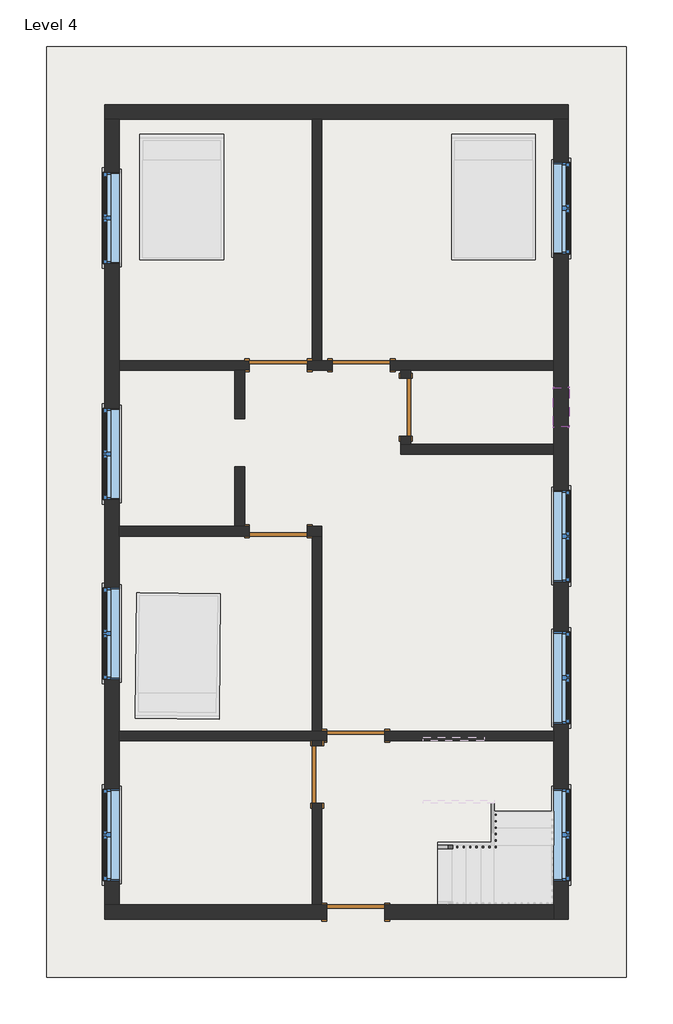
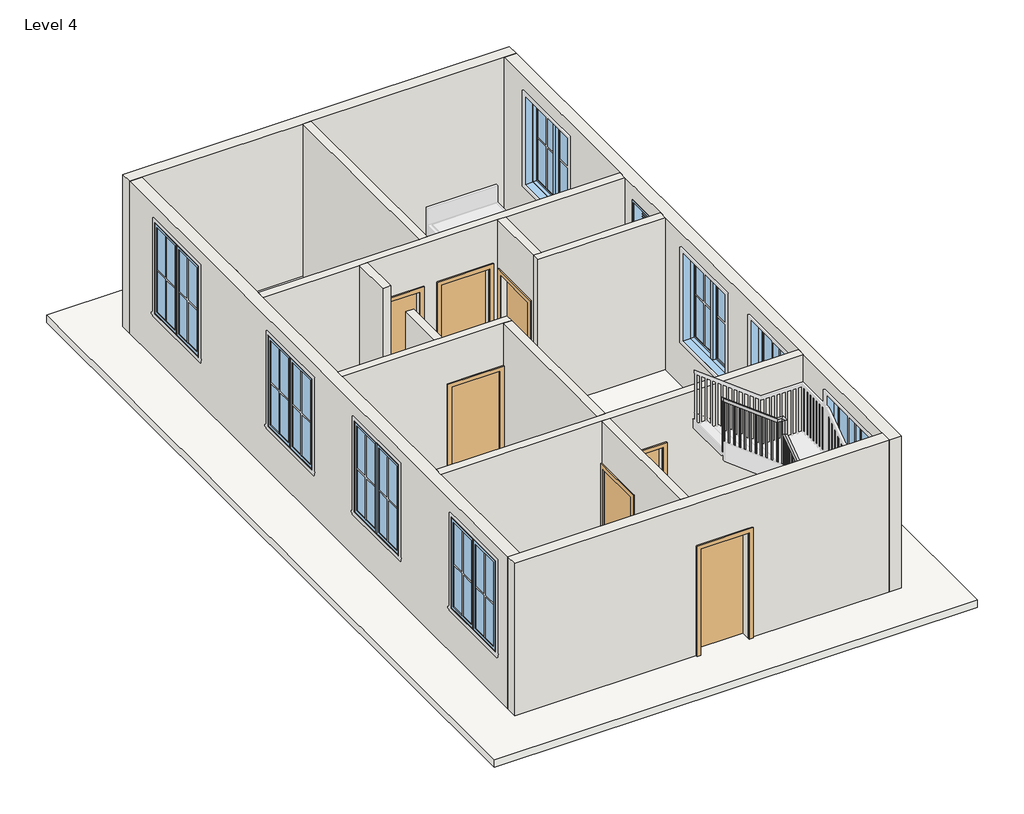
# One storey, part 1 of 2: 14 walls, 9 windows, 7 doors, 1 railing, 1 roof.
"""IFC4 building model written with IfcOpenShell, lengths in millimetres."""

from ifc_helpers import new_model, si_unit, frame, origin, place, context, project, spatial, polyline, outline, extrude, faceted_brep, transform, mapped, element, save
from components import door_2b0b55a0, door_686f89d2, door_16372e1c, door_a90ba1ad, window_9ac97e1a, window_f2d8fef0

model = new_model("IFC4")

# Units and contexts
model_context = context("Model", 3, world=origin())
ifc_project = project(units=[si_unit("LENGTHUNIT", "METRE", prefix="MILLI")], contexts=[model_context])

# Site, building, storey
site = spatial("IfcSite", under=ifc_project)
building = spatial("IfcBuilding", under=site)
storey = spatial("IfcBuildingStorey", under=building, Name="Level 4", Elevation=6400.8)

# Doors
placement = place(None, origin())
door_shape = door_2b0b55a0(model_context)
element("IfcDoor", 1, ObjectType="Single-Flush : 36\" x 80\"", at=placement, inside=storey, context=model_context, shape_type="MappedRepresentation", body=[
    mapped(door_shape, transform((-163.235885, 1707.4649429, 6400.8), x_axis=(0.0, 1.0, 0.0), y_axis=(-1.0, 0.0, 0.0), z_axis=(0.0, 0.0, 1.0))),
])
door_2_shape = door_686f89d2(model_context)
element("IfcDoor", 2, ObjectType="Single-Flush : 36\" x 84\"", at=placement, inside=storey, context=model_context, shape_type="MappedRepresentation", body=[
    mapped(door_2_shape, transform((-861.735885, 2367.8649429, 6400.8), x_axis=(-1.0, 0.0, 0.0), y_axis=(0.0, -1.0, 0.0), z_axis=(0.0, 0.0, 1.0))),
])
element("IfcDoor", 3, ObjectType="Single-Flush : 36\" x 84\"", at=placement, inside=storey, context=model_context, shape_type="MappedRepresentation", body=[
    mapped(door_2_shape, transform((-2169.835885, -248.3350571, 6400.8), x_axis=(1.0, 0.0, 0.0), y_axis=(0.0, 1.0, 0.0), z_axis=(0.0, 0.0, 1.0))),
])
element("IfcDoor", 4, ObjectType="Single-Flush : 36\" x 84\"", at=placement, inside=storey, context=model_context, shape_type="MappedRepresentation", body=[
    mapped(door_2_shape, transform((-950.635885, -3474.1350571, 6400.8), x_axis=(-1.0, 0.0, 0.0), y_axis=(0.0, -1.0, 0.0), z_axis=(0.0, 0.0, 1.0))),
])
door_3_shape = door_16372e1c(model_context)
element("IfcDoor", 5, ObjectType="Single-Flush : 36\" x 84\"", at=placement, inside=storey, context=model_context, shape_type="MappedRepresentation", body=[
    mapped(door_3_shape, transform((-2169.835885, 2367.8649429, 6400.8), x_axis=(1.0, 0.0, 0.0), y_axis=(0.0, 1.0, 0.0), z_axis=(0.0, 0.0, 1.0))),
])
element("IfcDoor", 6, ObjectType="Single-Flush : 36\" x 84\"", at=placement, inside=storey, context=model_context, shape_type="MappedRepresentation", body=[
    mapped(door_3_shape, transform((-1560.235885, -4083.7350571, 6400.8), x_axis=(0.0, 1.0, 0.0), y_axis=(-1.0, 0.0, 0.0), z_axis=(0.0, 0.0, 1.0))),
])
door_4_shape = door_a90ba1ad(model_context)
element("IfcDoor", 7, ObjectType="Single-Flush : 36\" x 84\"", at=placement, inside=storey, context=model_context, shape_type="MappedRepresentation", body=[
    mapped(door_4_shape, transform((-950.635885, -6255.4350571, 6400.8), x_axis=(-1.0, 0.0, 0.0), y_axis=(0.0, -1.0, 0.0), z_axis=(0.0, 0.0, 1.0))),
])

# Railing
element("IfcRailing", 8, ObjectType="Handrail - Rectangular", at=placement, inside=storey, context=model_context, shape_type="SolidModel", body=[
    faceted_brep([(344.764115, -5201.3350571, 7484.5333333), (344.764115, -5201.3350571, 7420.6686436), (344.764115, -5252.1350571, 7420.6686436), (344.764115, -5252.1350571, 7484.5333333), (1157.564115, -5201.3350571, 8103.8095238), (1208.364115, -5201.3350571, 8078.649596), (1208.364115, -5252.1350571, 8078.649596), (1157.564115, -5252.1350571, 8103.8095238), (1157.564115, -5201.3350571, 8385.6285714), (1208.364115, -5201.3350571, 8334.8285714), (1208.364115, -5252.1350571, 8334.8285714), (1157.564115, -5252.1350571, 8385.6285714), (1233.764115, -5201.3350571, 8385.6285714), (1233.764115, -5201.3350571, 8334.8285714), (1284.564115, -5252.1350571, 8334.8285714), (1284.564115, -5252.1350571, 8385.6285714), (1233.764115, -5125.1350571, 8385.6285714), (1233.764115, -5108.8554323, 8334.8285714), (1284.564115, -5108.8554323, 8334.8285714), (1284.564115, -5125.1350571, 8385.6285714), (1233.764115, -4566.3350571, 8784.7714286), (1233.764115, -4515.5350571, 8758.6288395), (1284.564115, -4515.5350571, 8758.6288395), (1284.564115, -4566.3350571, 8784.7714286), (1233.764115, -4566.3350571, 9066.2606061), (1233.764115, -4515.5350571, 9015.4606061), (1284.564115, -4515.5350571, 9015.4606061), (1284.564115, -4566.3350571, 9066.2606061), (1233.764115, -4490.1350571, 9066.2606061), (1233.764115, -4490.1350571, 9015.4606061), (1284.564115, -4439.3350571, 9015.4606061), (1284.564115, -4439.3350571, 9066.2606061), (1157.564115, -4490.1350571, 9066.2606061), (1140.4943334, -4490.1350571, 9015.4606061), (1140.4943334, -4439.3350571, 9015.4606061), (1157.564115, -4439.3350571, 9066.2606061), (116.164115, -4490.1350571, 9855.2), (116.164115, -4439.3350571, 9855.2), (116.164115, -4439.3350571, 9791.4683472), (116.164115, -4490.1350571, 9791.4683472)], [[[0, 1, 2, 3]], [[1, 0, 4, 5]], [[2, 1, 5, 6]], [[3, 2, 6, 7]], [[0, 3, 7, 4]], [[5, 4, 8, 9]], [[6, 5, 9, 10]], [[7, 6, 10, 11]], [[4, 7, 11, 8]], [[9, 8, 12, 13]], [[10, 9, 13, 14]], [[11, 10, 14, 15]], [[8, 11, 15, 12]], [[13, 12, 16, 17]], [[14, 13, 17, 18]], [[15, 14, 18, 19]], [[12, 15, 19, 16]], [[17, 16, 20, 21]], [[18, 17, 21, 22]], [[19, 18, 22, 23]], [[16, 19, 23, 20]], [[21, 20, 24, 25]], [[22, 21, 25, 26]], [[23, 22, 26, 27]], [[20, 23, 27, 24]], [[25, 24, 28, 29]], [[26, 25, 29, 30]], [[27, 26, 30, 31]], [[24, 27, 31, 28]], [[29, 28, 32, 33]], [[30, 29, 33, 34]], [[31, 30, 34, 35]], [[28, 31, 35, 32]], [[36, 37, 38, 39]], [[33, 32, 36, 39]], [[34, 33, 39, 38]], [[35, 34, 38, 37]], [[32, 35, 37, 36]]]),
    extrude(outline(polyline([(9779.4418321, 132.039115), (8771.4666667, 132.039115), (8771.4666667, 151.089115), (9765.0100139, 151.089115), (9779.4418321, 132.039115)])), frame((0.0, -4474.2600571, 0.0), z_axis=(0.0, 1.0, 0.0), x_axis=(0.0, 0.0, 1.0)), (0.0, 0.0, 1.0), 19.05),
    extrude(outline(polyline([(9702.4721351, 233.639115), (8771.4666667, 233.639115), (8771.4666667, 252.689115), (9688.0403169, 252.689115), (9702.4721351, 233.639115)])), frame((0.0, -4474.2600571, 0.0), z_axis=(0.0, 1.0, 0.0), x_axis=(0.0, 0.0, 1.0)), (0.0, 0.0, 1.0), 19.05),
    extrude(outline(polyline([(9625.5024382, 335.239115), (8771.4666667, 335.239115), (8771.4666667, 354.289115), (9611.07062, 354.289115), (9625.5024382, 335.239115)])), frame((0.0, -4474.2600571, 0.0), z_axis=(0.0, 1.0, 0.0), x_axis=(0.0, 0.0, 1.0)), (0.0, 0.0, 1.0), 19.05),
    extrude(outline(polyline([(9548.5327412, 436.839115), (8602.1333333, 436.839115), (8602.1333333, 455.889115), (9534.100923, 455.889115), (9548.5327412, 436.839115)])), frame((0.0, -4474.2600571, 0.0), z_axis=(0.0, 1.0, 0.0), x_axis=(0.0, 0.0, 1.0)), (0.0, 0.0, 1.0), 19.05),
    extrude(outline(polyline([(9471.5630442, 538.439115), (8602.1333333, 538.439115), (8602.1333333, 557.489115), (9457.131226, 557.489115), (9471.5630442, 538.439115)])), frame((0.0, -4474.2600571, 0.0), z_axis=(0.0, 1.0, 0.0), x_axis=(0.0, 0.0, 1.0)), (0.0, 0.0, 1.0), 19.05),
    extrude(outline(polyline([(9394.5933472, 640.039115), (8432.8, 640.039115), (8432.8, 659.089115), (9380.1615291, 659.089115), (9394.5933472, 640.039115)])), frame((0.0, -4474.2600571, 0.0), z_axis=(0.0, 1.0, 0.0), x_axis=(0.0, 0.0, 1.0)), (0.0, 0.0, 1.0), 19.05),
    extrude(outline(polyline([(9317.6236503, 741.639115), (8432.8, 741.639115), (8432.8, 760.689115), (9303.1918321, 760.689115), (9317.6236503, 741.639115)])), frame((0.0, -4474.2600571, 0.0), z_axis=(0.0, 1.0, 0.0), x_axis=(0.0, 0.0, 1.0)), (0.0, 0.0, 1.0), 19.05),
    extrude(outline(polyline([(9240.6539533, 843.239115), (8263.4666667, 843.239115), (8263.4666667, 862.289115), (9226.2221351, 862.289115), (9240.6539533, 843.239115)])), frame((0.0, -4474.2600571, 0.0), z_axis=(0.0, 1.0, 0.0), x_axis=(0.0, 0.0, 1.0)), (0.0, 0.0, 1.0), 19.05),
    extrude(outline(polyline([(9163.6842563, 944.839115), (8263.4666667, 944.839115), (8263.4666667, 963.889115), (9149.2524382, 963.889115), (9163.6842563, 944.839115)])), frame((0.0, -4474.2600571, 0.0), z_axis=(0.0, 1.0, 0.0), x_axis=(0.0, 0.0, 1.0)), (0.0, 0.0, 1.0), 19.05),
    extrude(outline(polyline([(9086.7145594, 1046.439115), (8094.1333333, 1046.439115), (8094.1333333, 1065.489115), (9072.2827412, 1065.489115), (9086.7145594, 1046.439115)])), frame((0.0, -4474.2600571, 0.0), z_axis=(0.0, 1.0, 0.0), x_axis=(0.0, 0.0, 1.0)), (0.0, 0.0, 1.0), 19.05),
    extrude(outline(polyline([(9009.7448624, 1148.039115), (8094.1333333, 1148.039115), (8094.1333333, 1167.089115), (8995.3130442, 1167.089115), (9009.7448624, 1148.039115)])), frame((0.0, -4474.2600571, 0.0), z_axis=(0.0, 1.0, 0.0), x_axis=(0.0, 0.0, 1.0)), (0.0, 0.0, 1.0), 19.05),
    extrude(outline(polyline([(1249.639115, -4525.0600571), (1249.639115, -4506.0100571), (1268.689115, -4506.0100571), (1268.689115, -4525.0600571), (1249.639115, -4525.0600571)])), frame((0.0, 0.0, 7755.4666667), z_axis=(0.0, 0.0, 1.0), x_axis=(1.0, 0.0, 0.0)), (0.0, 0.0, 1.0), 1259.9939394),
    extrude(outline(polyline([(-4607.6100571, 8692.8609823), (-4607.6100571, 7755.4666667), (-4626.6600571, 7755.4666667), (-4626.6600571, 8679.2538395), (-4607.6100571, 8692.8609823)])), frame((1249.639115, 0.0, 0.0), z_axis=(1.0, 0.0, 0.0), x_axis=(0.0, 1.0, 0.0)), (0.0, 0.0, 1.0), 19.05),
    extrude(outline(polyline([(-4709.2100571, 8620.2895538), (-4709.2100571, 7586.1333333), (-4728.2600571, 7586.1333333), (-4728.2600571, 8606.6824109), (-4709.2100571, 8620.2895538)])), frame((1249.639115, 0.0, 0.0), z_axis=(1.0, 0.0, 0.0), x_axis=(0.0, 1.0, 0.0)), (0.0, 0.0, 1.0), 19.05),
    extrude(outline(polyline([(-4810.8100571, 8547.7181252), (-4810.8100571, 7586.1333333), (-4829.8600571, 7586.1333333), (-4829.8600571, 8534.1109823), (-4810.8100571, 8547.7181252)])), frame((1249.639115, 0.0, 0.0), z_axis=(1.0, 0.0, 0.0), x_axis=(0.0, 1.0, 0.0)), (0.0, 0.0, 1.0), 19.05),
    extrude(outline(polyline([(-4912.4100571, 8475.1466966), (-4912.4100571, 7586.1333333), (-4931.4600571, 7586.1333333), (-4931.4600571, 8461.5395538), (-4912.4100571, 8475.1466966)])), frame((1249.639115, 0.0, 0.0), z_axis=(1.0, 0.0, 0.0), x_axis=(0.0, 1.0, 0.0)), (0.0, 0.0, 1.0), 19.05),
    extrude(outline(polyline([(-5014.0100571, 8402.5752681), (-5014.0100571, 7416.8), (-5033.0600571, 7416.8), (-5033.0600571, 8388.9681252), (-5014.0100571, 8402.5752681)])), frame((1249.639115, 0.0, 0.0), z_axis=(1.0, 0.0, 0.0), x_axis=(0.0, 1.0, 0.0)), (0.0, 0.0, 1.0), 19.05),
    extrude(outline(polyline([(-5115.6100571, 8330.0038395), (-5115.6100571, 7416.8), (-5134.6600571, 7416.8), (-5134.6600571, 8316.3966966), (-5115.6100571, 8330.0038395)])), frame((1249.639115, 0.0, 0.0), z_axis=(1.0, 0.0, 0.0), x_axis=(0.0, 1.0, 0.0)), (0.0, 0.0, 1.0), 19.05),
    extrude(outline(polyline([(8032.6876912, 1148.039115), (7078.1333333, 1148.039115), (7078.1333333, 1167.089115), (8047.2019769, 1167.089115), (8032.6876912, 1148.039115)])), frame((0.0, -5236.2600571, 0.0), z_axis=(0.0, 1.0, 0.0), x_axis=(0.0, 0.0, 1.0)), (0.0, 0.0, 1.0), 19.05),
    extrude(outline(polyline([(7955.2781674, 1046.439115), (7078.1333333, 1046.439115), (7078.1333333, 1065.489115), (7969.7924531, 1065.489115), (7955.2781674, 1046.439115)])), frame((0.0, -5236.2600571, 0.0), z_axis=(0.0, 1.0, 0.0), x_axis=(0.0, 0.0, 1.0)), (0.0, 0.0, 1.0), 19.05),
    extrude(outline(polyline([(7877.8686436, 944.839115), (6908.8, 944.839115), (6908.8, 963.889115), (7892.3829293, 963.889115), (7877.8686436, 944.839115)])), frame((0.0, -5236.2600571, 0.0), z_axis=(0.0, 1.0, 0.0), x_axis=(0.0, 0.0, 1.0)), (0.0, 0.0, 1.0), 19.05),
    extrude(outline(polyline([(7800.4591198, 843.239115), (6908.8, 843.239115), (6908.8, 862.289115), (7814.9734055, 862.289115), (7800.4591198, 843.239115)])), frame((0.0, -5236.2600571, 0.0), z_axis=(0.0, 1.0, 0.0), x_axis=(0.0, 0.0, 1.0)), (0.0, 0.0, 1.0), 19.05),
    extrude(outline(polyline([(7723.049596, 741.639115), (6739.4666667, 741.639115), (6739.4666667, 760.689115), (7737.5638817, 760.689115), (7723.049596, 741.639115)])), frame((0.0, -5236.2600571, 0.0), z_axis=(0.0, 1.0, 0.0), x_axis=(0.0, 0.0, 1.0)), (0.0, 0.0, 1.0), 19.05),
    extrude(outline(polyline([(7645.6400722, 640.039115), (6739.4666667, 640.039115), (6739.4666667, 659.089115), (7660.1543579, 659.089115), (7645.6400722, 640.039115)])), frame((0.0, -5236.2600571, 0.0), z_axis=(0.0, 1.0, 0.0), x_axis=(0.0, 0.0, 1.0)), (0.0, 0.0, 1.0), 19.05),
    extrude(outline(polyline([(7568.2305484, 538.439115), (6570.1333333, 538.439115), (6570.1333333, 557.489115), (7582.7448341, 557.489115), (7568.2305484, 538.439115)])), frame((0.0, -5236.2600571, 0.0), z_axis=(0.0, 1.0, 0.0), x_axis=(0.0, 0.0, 1.0)), (0.0, 0.0, 1.0), 19.05),
    extrude(outline(polyline([(7490.8210246, 436.839115), (6570.1333333, 436.839115), (6570.1333333, 455.889115), (7505.3353103, 455.889115), (7490.8210246, 436.839115)])), frame((0.0, -5236.2600571, 0.0), z_axis=(0.0, 1.0, 0.0), x_axis=(0.0, 0.0, 1.0)), (0.0, 0.0, 1.0), 19.05),
    extrude(outline(polyline([(1249.639115, -4474.2600571), (1249.639115, -4455.2100571), (1268.689115, -4455.2100571), (1268.689115, -4474.2600571), (1249.639115, -4474.2600571)])), frame((0.0, 0.0, 7924.8), z_axis=(0.0, 0.0, 1.0), x_axis=(1.0, 0.0, 0.0)), (0.0, 0.0, 1.0), 1090.6606061),
    extrude(outline(polyline([(1249.639115, -5217.2100571), (1268.689115, -5217.2100571), (1268.689115, -5236.2600571), (1249.639115, -5236.2600571), (1249.639115, -5217.2100571)])), frame((0.0, 0.0, 7247.4666667), z_axis=(0.0, 0.0, 1.0), x_axis=(1.0, 0.0, 0.0)), (0.0, 0.0, 1.0), 1087.3619048),
    extrude(outline(polyline([(9791.4683472, 116.164115), (8771.4666667, 116.164115), (8771.4666667, 135.214115), (9777.0365291, 135.214115), (9791.4683472, 116.164115)])), frame((0.0, -4474.2600571, 0.0), z_axis=(0.0, 1.0, 0.0), x_axis=(0.0, 0.0, 1.0)), (0.0, 0.0, 1.0), 19.05),
    extrude(outline(polyline([(7420.6686436, 344.764115), (6570.1333333, 344.764115), (6570.1333333, 363.814115), (7435.1829293, 363.814115), (7420.6686436, 344.764115)])), frame((0.0, -5236.2600571, 0.0), z_axis=(0.0, 1.0, 0.0), x_axis=(0.0, 0.0, 1.0)), (0.0, 0.0, 1.0), 19.05),
])

# Roof
element("IfcRoof", 9, ObjectType="ROOF 6\"", at=placement, inside=storey, context=model_context, shape_type="SweptSolid", body=[
    extrude(outline(polyline([(-5827.435885, 7397.0649429), (3316.564115, 7397.0649429), (3316.564115, -7284.1350571), (-5827.435885, -7284.1350571), (-5827.435885, 7397.0649429)])), frame((0.0, 0.0, 6248.4), z_axis=(0.0, 0.0, 1.0), x_axis=(1.0, 0.0, 0.0)), (0.0, 0.0, 1.0), 152.4),
])

# Walls
element("IfcWall", 10, ObjectType="WALL 6\"", at=placement, inside=storey, context=model_context, shape_type="SweptSolid", body=[
    extrude(outline(polyline([(-1636.435885, 2444.0649429), (-1636.435885, 6254.0649429), (-1484.035885, 6254.0649429), (-1484.035885, 2444.0649429), (-1636.435885, 2444.0649429)])), frame((0.0, 0.0, 6400.8), z_axis=(0.0, 0.0, 1.0), x_axis=(1.0, 0.0, 0.0)), (0.0, 0.0, 1.0), 3048.0),
])
element("IfcWall", 11, ObjectType="WALL 6\"", at=placement, inside=storey, context=model_context, shape_type="Brep", body=[
    faceted_brep([(-1318.935885, 2444.0649429, 6400.8), (-1484.035885, 2444.0649429, 6400.8), (-1636.435885, 2444.0649429, 6400.8), (-1712.635885, 2444.0649429, 6400.8), (-1712.635885, 2444.0649429, 8534.4), (-2627.035885, 2444.0649429, 8534.4), (-2627.035885, 2444.0649429, 6400.8), (-4684.435885, 2444.0649429, 6400.8), (-4684.435885, 2444.0649429, 9448.8), (-1636.435885, 2444.0649429, 9448.8), (-1484.035885, 2444.0649429, 9448.8), (2173.564115, 2444.0649429, 9448.8), (2173.564115, 2444.0649429, 6400.8), (-404.535885, 2444.0649429, 6400.8), (-404.535885, 2444.0649429, 8534.4), (-1318.935885, 2444.0649429, 8534.4), (-1712.635885, 2291.6649429, 8534.4), (-1712.635885, 2291.6649429, 6400.8), (-1318.935885, 2291.6649429, 6400.8), (-1318.935885, 2291.6649429, 8534.4), (-404.535885, 2291.6649429, 8534.4), (-404.535885, 2291.6649429, 6400.8), (-239.435885, 2291.6649429, 6400.8), (-87.035885, 2291.6649429, 6400.8), (2173.564115, 2291.6649429, 6400.8), (2173.564115, 2291.6649429, 9448.8), (-87.035885, 2291.6649429, 9448.8), (-239.435885, 2291.6649429, 9448.8), (-2703.235885, 2291.6649429, 9448.8), (-2855.635885, 2291.6649429, 9448.8), (-4684.435885, 2291.6649429, 9448.8), (-4684.435885, 2291.6649429, 6400.8), (-2855.635885, 2291.6649429, 6400.8), (-2703.235885, 2291.6649429, 6400.8), (-2627.035885, 2291.6649429, 6400.8), (-2627.035885, 2291.6649429, 8534.4)], [[[0, 1, 2, 3, 4, 5, 6, 7, 8, 9, 10, 11, 12, 13, 14, 15]], [[16, 17, 18, 19, 20, 21, 22, 23, 24, 25, 26, 27, 28, 29, 30, 31, 32, 33, 34, 35]], [[13, 12, 24, 23, 22, 21]], [[18, 17, 3, 2, 1, 0]], [[34, 33, 32, 31, 7, 6]], [[12, 11, 25, 24]], [[8, 7, 31, 30]], [[19, 18, 0, 15]], [[20, 19, 15, 14]], [[21, 20, 14, 13]], [[4, 3, 17, 16]], [[5, 4, 16, 35]], [[6, 5, 35, 34]], [[11, 10, 9, 8, 30, 29, 28, 27, 26, 25]]]),
])
element("IfcWall", 12, ObjectType="WALL 6\"", at=placement, inside=storey, context=model_context, shape_type="SweptSolid", body=[
    extrude(outline(polyline([(-2855.635885, 1529.6649429), (-2855.635885, 2291.6649429), (-2703.235885, 2291.6649429), (-2703.235885, 1529.6649429), (-2855.635885, 1529.6649429)])), frame((0.0, 0.0, 6400.8), z_axis=(0.0, 0.0, 1.0), x_axis=(1.0, 0.0, 0.0)), (0.0, 0.0, 1.0), 3048.0),
])
element("IfcWall", 13, ObjectType="WALL 6\"", at=placement, inside=storey, context=model_context, shape_type="Brep", body=[
    faceted_brep([(-1712.635885, -324.5350571, 8534.4), (-1712.635885, -324.5350571, 6400.8), (-1636.435885, -324.5350571, 6400.8), (-1484.035885, -324.5350571, 6400.8), (-1484.035885, -324.5350571, 9448.8), (-1636.435885, -324.5350571, 9448.8), (-4684.435885, -324.5350571, 9448.8), (-4684.435885, -324.5350571, 6400.8), (-2627.035885, -324.5350571, 6400.8), (-2627.035885, -324.5350571, 8534.4), (-1484.035885, -172.1350571, 6400.8), (-1712.635885, -172.1350571, 6400.8), (-1712.635885, -172.1350571, 8534.4), (-2627.035885, -172.1350571, 8534.4), (-2627.035885, -172.1350571, 6400.8), (-2703.235885, -172.1350571, 6400.8), (-2855.635885, -172.1350571, 6400.8), (-4684.435885, -172.1350571, 6400.8), (-4684.435885, -172.1350571, 9448.8), (-2855.635885, -172.1350571, 9448.8), (-2703.235885, -172.1350571, 9448.8), (-1484.035885, -172.1350571, 9448.8)], [[[0, 1, 2, 3, 4, 5, 6, 7, 8, 9]], [[10, 11, 12, 13, 14, 15, 16, 17, 18, 19, 20, 21]], [[8, 7, 17, 16, 15, 14]], [[3, 2, 1, 11, 10]], [[7, 6, 18, 17]], [[4, 3, 10, 21]], [[12, 11, 1, 0]], [[13, 12, 0, 9]], [[14, 13, 9, 8]], [[6, 5, 4, 21, 20, 19, 18]]]),
])
element("IfcWall", 14, ObjectType="WALL 6\"", at=placement, inside=storey, context=model_context, shape_type="SweptSolid", body=[
    extrude(outline(polyline([(-1636.435885, -3397.9350571), (-1636.435885, -324.5350571), (-1484.035885, -324.5350571), (-1484.035885, -3397.9350571), (-1636.435885, -3397.9350571)])), frame((0.0, 0.0, 6400.8), z_axis=(0.0, 0.0, 1.0), x_axis=(1.0, 0.0, 0.0)), (0.0, 0.0, 1.0), 3048.0),
])
element("IfcWall", 15, ObjectType="WALL 6\"", at=placement, inside=storey, context=model_context, shape_type="Brep", body=[
    faceted_brep([(-4684.435885, -3550.3350571, 6400.8), (-1636.435885, -3550.3350571, 6400.8), (-1484.035885, -3550.3350571, 6400.8), (-1407.835885, -3550.3350571, 6400.8), (-1407.835885, -3550.3350571, 8534.4), (-493.435885, -3550.3350571, 8534.4), (-493.435885, -3550.3350571, 6400.8), (2173.564115, -3550.3350571, 6400.8), (2173.564115, -3550.3350571, 9448.8), (-1484.035885, -3550.3350571, 9448.8), (-1636.435885, -3550.3350571, 9448.8), (-4684.435885, -3550.3350571, 9448.8), (-1407.835885, -3397.9350571, 8534.4), (-1407.835885, -3397.9350571, 6400.8), (-1484.035885, -3397.9350571, 6400.8), (-1636.435885, -3397.9350571, 6400.8), (-4684.435885, -3397.9350571, 6400.8), (-4684.435885, -3397.9350571, 9448.8), (-1636.435885, -3397.9350571, 9448.8), (-1484.035885, -3397.9350571, 9448.8), (2173.564115, -3397.9350571, 9448.8), (2173.564115, -3397.9350571, 6400.8), (-493.435885, -3397.9350571, 6400.8), (-493.435885, -3397.9350571, 8534.4)], [[[0, 1, 2, 3, 4, 5, 6, 7, 8, 9, 10, 11]], [[12, 13, 14, 15, 16, 17, 18, 19, 20, 21, 22, 23]], [[22, 21, 7, 6]], [[16, 15, 14, 13, 3, 2, 1, 0]], [[8, 7, 21, 20]], [[0, 11, 17, 16]], [[4, 3, 13, 12]], [[5, 4, 12, 23]], [[6, 5, 23, 22]], [[11, 10, 9, 8, 20, 19, 18, 17]]]),
])
element("IfcWall", 16, ObjectType="WALL 6\"", at=placement, inside=storey, context=model_context, shape_type="SweptSolid", body=[
    extrude(outline(polyline([(-3550.3350571, 6400.8), (-3626.5350571, 6400.8), (-3626.5350571, 8534.4), (-4540.9350571, 8534.4), (-4540.9350571, 6400.8), (-6141.1350571, 6400.8), (-6141.1350571, 9448.8), (-3550.3350571, 9448.8), (-3550.3350571, 6400.8)])), frame((-1636.435885, 0.0, 0.0), z_axis=(1.0, 0.0, 0.0), x_axis=(0.0, 1.0, 0.0)), (0.0, 0.0, 1.0), 152.4),
])
element("IfcWall", 17, ObjectType="WALL 6\"", at=placement, inside=storey, context=model_context, shape_type="Brep", body=[
    faceted_brep([(2173.564115, 1123.2649429, 6400.8), (-87.035885, 1123.2649429, 6400.8), (-239.435885, 1123.2649429, 6400.8), (-239.435885, 1123.2649429, 9448.8), (-87.035885, 1123.2649429, 9448.8), (2173.564115, 1123.2649429, 9448.8), (2173.564115, 970.8649429, 6400.8), (2173.564115, 970.8649429, 9448.8), (-239.435885, 970.8649429, 9448.8), (-239.435885, 970.8649429, 6400.8)], [[[0, 1, 2, 3, 4, 5]], [[6, 7, 8, 9]], [[2, 1, 0, 6, 9]], [[0, 5, 7, 6]], [[3, 2, 9, 8]], [[5, 4, 3, 8, 7]]]),
])
element("IfcWall", 18, ObjectType="WALL 6\"", at=placement, inside=storey, context=model_context, shape_type="SweptSolid", body=[
    extrude(outline(polyline([(2291.6649429, 6400.8), (2164.6649429, 6400.8), (2164.6649429, 8432.8), (1250.2649429, 8432.8), (1250.2649429, 6400.8), (1123.2649429, 6400.8), (1123.2649429, 9448.8), (2291.6649429, 9448.8), (2291.6649429, 6400.8)])), frame((-239.435885, 0.0, 0.0), z_axis=(1.0, 0.0, 0.0), x_axis=(0.0, 1.0, 0.0)), (0.0, 0.0, 1.0), 152.4),
])
element("IfcWall", 19, ObjectType="WALL 6\"", at=placement, inside=storey, context=model_context, shape_type="SweptSolid", body=[
    extrude(outline(polyline([(-2855.635885, -172.1350571), (-2855.635885, 767.6649429), (-2703.235885, 767.6649429), (-2703.235885, -172.1350571), (-2855.635885, -172.1350571)])), frame((0.0, 0.0, 6400.8), z_axis=(0.0, 0.0, 1.0), x_axis=(1.0, 0.0, 0.0)), (0.0, 0.0, 1.0), 3048.0),
])
element("IfcWall", 20, ObjectType="WALL 9\"", at=placement, inside=storey, context=model_context, shape_type="Brep", body=[
    faceted_brep([(-4913.035885, 6254.0649429, 6400.8), (-4684.435885, 6254.0649429, 6400.8), (-1636.435885, 6254.0649429, 6400.8), (-1484.035885, 6254.0649429, 6400.8), (2173.564115, 6254.0649429, 6400.8), (2402.164115, 6254.0649429, 6400.8), (2402.164115, 6254.0649429, 9448.8), (2173.564115, 6254.0649429, 9448.8), (-1484.035885, 6254.0649429, 9448.8), (-1636.435885, 6254.0649429, 9448.8), (-4684.435885, 6254.0649429, 9448.8), (-4913.035885, 6254.0649429, 9448.8), (-4913.035885, 6482.6649429, 6400.8), (-4913.035885, 6482.6649429, 9448.8), (2402.164115, 6482.6649429, 9448.8), (2402.164115, 6482.6649429, 6400.8)], [[[0, 1, 2, 3, 4, 5, 6, 7, 8, 9, 10, 11]], [[12, 13, 14, 15]], [[5, 4, 3, 2, 1, 0, 12, 15]], [[6, 5, 15, 14]], [[0, 11, 13, 12]], [[11, 10, 9, 8, 7, 6, 14, 13]]]),
])
element("IfcWall", 21, ObjectType="WALL 9\"", at=placement, inside=storey, context=model_context, shape_type="Brep", body=[
    faceted_brep([(2173.564115, 6254.0649429, 6400.8), (2173.564115, 2444.0649429, 6400.8), (2173.564115, 2291.6649429, 6400.8), (2173.564115, 1123.2649429, 6400.8), (2173.564115, 970.8649429, 6400.8), (2173.564115, -3397.9350571, 6400.8), (2173.564115, -3550.3350571, 6400.8), (2173.564115, -6141.1350571, 6400.8), (2173.564115, -6369.7350571, 6400.8), (2173.564115, -6369.7350571, 9448.8), (2173.564115, -6141.1350571, 9448.8), (2173.564115, -3550.3350571, 9448.8), (2173.564115, -3397.9350571, 9448.8), (2173.564115, 970.8649429, 9448.8), (2173.564115, 1123.2649429, 9448.8), (2173.564115, 2291.6649429, 9448.8), (2173.564115, 2444.0649429, 9448.8), (2173.564115, 6254.0649429, 9448.8), (2173.564115, -5760.1350571, 9144.0), (2173.564115, -5760.1350571, 7315.2), (2173.564115, -4312.3350571, 7315.2), (2173.564115, -4312.3350571, 9144.0), (2173.564115, -3283.6350571, 9144.0), (2173.564115, -3283.6350571, 7315.2), (2173.564115, -1835.8350571, 7315.2), (2173.564115, -1835.8350571, 9144.0), (2173.564115, -1048.4350571, 9144.0), (2173.564115, -1048.4350571, 7315.2), (2173.564115, 399.3649429, 7315.2), (2173.564115, 399.3649429, 9144.0), (2173.564115, 4120.4649429, 9144.0), (2173.564115, 4120.4649429, 7315.2), (2173.564115, 5568.2649429, 7315.2), (2173.564115, 5568.2649429, 9144.0), (2173.564115, 2012.2649429, 9144.0), (2173.564115, 1402.6649429, 9144.0), (2173.564115, 1402.6649429, 8534.4), (2173.564115, 2012.2649429, 8534.4), (2402.164115, 6254.0649429, 6400.8), (2402.164115, 6254.0649429, 9448.8), (2402.164115, -6369.7350571, 9448.8), (2402.164115, -6369.7350571, 6400.8), (2402.164115, -5760.1350571, 9144.0), (2402.164115, -4312.3350571, 9144.0), (2402.164115, -4312.3350571, 7315.2), (2402.164115, -5760.1350571, 7315.2), (2402.164115, -3283.6350571, 9144.0), (2402.164115, -1835.8350571, 9144.0), (2402.164115, -1835.8350571, 7315.2), (2402.164115, -3283.6350571, 7315.2), (2402.164115, -1048.4350571, 9144.0), (2402.164115, 399.3649429, 9144.0), (2402.164115, 399.3649429, 7315.2), (2402.164115, -1048.4350571, 7315.2), (2402.164115, 4120.4649429, 9144.0), (2402.164115, 5568.2649429, 9144.0), (2402.164115, 5568.2649429, 7315.2), (2402.164115, 4120.4649429, 7315.2), (2402.164115, 2012.2649429, 9144.0), (2402.164115, 2012.2649429, 8534.4), (2402.164115, 1402.6649429, 8534.4), (2402.164115, 1402.6649429, 9144.0)], [[[0, 1, 2, 3, 4, 5, 6, 7, 8, 9, 10, 11, 12, 13, 14, 15, 16, 17], [18, 19, 20, 21], [22, 23, 24, 25], [26, 27, 28, 29], [30, 31, 32, 33], [34, 35, 36, 37]], [[38, 39, 40, 41], [42, 43, 44, 45], [46, 47, 48, 49], [50, 51, 52, 53], [54, 55, 56, 57], [58, 59, 60, 61]], [[8, 7, 6, 5, 4, 3, 2, 1, 0, 38, 41]], [[0, 17, 39, 38]], [[9, 8, 41, 40]], [[19, 18, 42, 45]], [[20, 19, 45, 44]], [[21, 20, 44, 43]], [[18, 21, 43, 42]], [[23, 22, 46, 49]], [[24, 23, 49, 48]], [[25, 24, 48, 47]], [[22, 25, 47, 46]], [[27, 26, 50, 53]], [[28, 27, 53, 52]], [[29, 28, 52, 51]], [[26, 29, 51, 50]], [[31, 30, 54, 57]], [[32, 31, 57, 56]], [[33, 32, 56, 55]], [[30, 33, 55, 54]], [[59, 58, 34, 37]], [[60, 59, 37, 36]], [[61, 60, 36, 35]], [[58, 61, 35, 34]], [[17, 16, 15, 14, 13, 12, 11, 10, 9, 40, 39]]]),
])
element("IfcWall", 22, ObjectType="WALL 9\"", at=placement, inside=storey, context=model_context, shape_type="Brep", body=[
    faceted_brep([(-1407.835885, -6141.1350571, 8534.4), (-1407.835885, -6141.1350571, 6400.8), (-1484.035885, -6141.1350571, 6400.8), (-1636.435885, -6141.1350571, 6400.8), (-4684.435885, -6141.1350571, 6400.8), (-4913.035885, -6141.1350571, 6400.8), (-4913.035885, -6141.1350571, 9448.8), (-4684.435885, -6141.1350571, 9448.8), (-1636.435885, -6141.1350571, 9448.8), (-1484.035885, -6141.1350571, 9448.8), (2173.564115, -6141.1350571, 9448.8), (2173.564115, -6141.1350571, 6400.8), (-493.435885, -6141.1350571, 6400.8), (-493.435885, -6141.1350571, 8534.4), (-4913.035885, -6369.7350571, 6400.8), (-1407.835885, -6369.7350571, 6400.8), (-1407.835885, -6369.7350571, 8534.4), (-493.435885, -6369.7350571, 8534.4), (-493.435885, -6369.7350571, 6400.8), (2173.564115, -6369.7350571, 6400.8), (2173.564115, -6369.7350571, 9448.8), (-4913.035885, -6369.7350571, 9448.8)], [[[0, 1, 2, 3, 4, 5, 6, 7, 8, 9, 10, 11, 12, 13]], [[14, 15, 16, 17, 18, 19, 20, 21]], [[12, 11, 19, 18]], [[5, 4, 3, 2, 1, 15, 14]], [[11, 10, 20, 19]], [[6, 5, 14, 21]], [[16, 15, 1, 0]], [[17, 16, 0, 13]], [[18, 17, 13, 12]], [[10, 9, 8, 7, 6, 21, 20]]]),
])
element("IfcWall", 23, ObjectType="WALL 9\"", at=placement, inside=storey, context=model_context, shape_type="Brep", body=[
    faceted_brep([(-4684.435885, -6141.1350571, 6400.8), (-4684.435885, -3550.3350571, 6400.8), (-4684.435885, -3397.9350571, 6400.8), (-4684.435885, -324.5350571, 6400.8), (-4684.435885, -172.1350571, 6400.8), (-4684.435885, 2291.6649429, 6400.8), (-4684.435885, 2444.0649429, 6400.8), (-4684.435885, 6254.0649429, 6400.8), (-4684.435885, 6254.0649429, 9448.8), (-4684.435885, 2444.0649429, 9448.8), (-4684.435885, 2291.6649429, 9448.8), (-4684.435885, -172.1350571, 9448.8), (-4684.435885, -324.5350571, 9448.8), (-4684.435885, -3397.9350571, 9448.8), (-4684.435885, -3550.3350571, 9448.8), (-4684.435885, -6141.1350571, 9448.8), (-4684.435885, -4312.3350571, 9144.0), (-4684.435885, -4312.3350571, 7315.2), (-4684.435885, -5760.1350571, 7315.2), (-4684.435885, -5760.1350571, 9144.0), (-4684.435885, -1137.3350571, 9144.0), (-4684.435885, -1137.3350571, 7315.2), (-4684.435885, -2585.1350571, 7315.2), (-4684.435885, -2585.1350571, 9144.0), (-4684.435885, 1694.7649429, 9144.0), (-4684.435885, 1694.7649429, 7315.2), (-4684.435885, 246.9649429, 7315.2), (-4684.435885, 246.9649429, 9144.0), (-4684.435885, 5415.8649429, 9144.0), (-4684.435885, 5415.8649429, 7315.2), (-4684.435885, 3968.0649429, 7315.2), (-4684.435885, 3968.0649429, 9144.0), (-4913.035885, -6141.1350571, 6400.8), (-4913.035885, -6141.1350571, 9448.8), (-4913.035885, 6254.0649429, 9448.8), (-4913.035885, 6254.0649429, 6400.8), (-4913.035885, -4312.3350571, 9144.0), (-4913.035885, -5760.1350571, 9144.0), (-4913.035885, -5760.1350571, 7315.2), (-4913.035885, -4312.3350571, 7315.2), (-4913.035885, -1137.3350571, 9144.0), (-4913.035885, -2585.1350571, 9144.0), (-4913.035885, -2585.1350571, 7315.2), (-4913.035885, -1137.3350571, 7315.2), (-4913.035885, 1694.7649429, 9144.0), (-4913.035885, 246.9649429, 9144.0), (-4913.035885, 246.9649429, 7315.2), (-4913.035885, 1694.7649429, 7315.2), (-4913.035885, 5415.8649429, 9144.0), (-4913.035885, 3968.0649429, 9144.0), (-4913.035885, 3968.0649429, 7315.2), (-4913.035885, 5415.8649429, 7315.2)], [[[0, 1, 2, 3, 4, 5, 6, 7, 8, 9, 10, 11, 12, 13, 14, 15], [16, 17, 18, 19], [20, 21, 22, 23], [24, 25, 26, 27], [28, 29, 30, 31]], [[32, 33, 34, 35], [36, 37, 38, 39], [40, 41, 42, 43], [44, 45, 46, 47], [48, 49, 50, 51]], [[7, 6, 5, 4, 3, 2, 1, 0, 32, 35]], [[8, 7, 35, 34]], [[0, 15, 33, 32]], [[17, 16, 36, 39]], [[18, 17, 39, 38]], [[19, 18, 38, 37]], [[16, 19, 37, 36]], [[21, 20, 40, 43]], [[22, 21, 43, 42]], [[23, 22, 42, 41]], [[20, 23, 41, 40]], [[25, 24, 44, 47]], [[26, 25, 47, 46]], [[27, 26, 46, 45]], [[24, 27, 45, 44]], [[29, 28, 48, 51]], [[30, 29, 51, 50]], [[31, 30, 50, 49]], [[28, 31, 49, 48]], [[15, 14, 13, 12, 11, 10, 9, 8, 34, 33]]]),
])

# Windows
window_shape = window_9ac97e1a(model_context)
element("IfcWindow", 24, ObjectType="Window-Casement-Double : 57\" x 72\"", at=placement, inside=storey, context=model_context, shape_type="MappedRepresentation", body=[
    mapped(window_shape, transform((-4798.735885, -5036.2350571, 6400.8), x_axis=(0.0, 1.0, 0.0), y_axis=(-1.0, 0.0, 0.0), z_axis=(0.0, 0.0, 1.0))),
])
element("IfcWindow", 25, ObjectType="Window-Casement-Double : 57\" x 72\"", at=placement, inside=storey, context=model_context, shape_type="MappedRepresentation", body=[
    mapped(window_shape, transform((2287.864115, -5036.2350571, 6400.8), x_axis=(0.0, -1.0, 0.0), y_axis=(1.0, 0.0, 0.0), z_axis=(0.0, 0.0, 1.0))),
])
element("IfcWindow", 26, ObjectType="Window-Casement-Double : 57\" x 72\"", at=placement, inside=storey, context=model_context, shape_type="MappedRepresentation", body=[
    mapped(window_shape, transform((2287.864115, -2559.7350571, 6400.8), x_axis=(0.0, -1.0, 0.0), y_axis=(1.0, 0.0, 0.0), z_axis=(0.0, 0.0, 1.0))),
])
element("IfcWindow", 27, ObjectType="Window-Casement-Double : 57\" x 72\"", at=placement, inside=storey, context=model_context, shape_type="MappedRepresentation", body=[
    mapped(window_shape, transform((2287.864115, -324.5350571, 6400.8), x_axis=(0.0, -1.0, 0.0), y_axis=(1.0, 0.0, 0.0), z_axis=(0.0, 0.0, 1.0))),
])
element("IfcWindow", 28, ObjectType="Window-Casement-Double : 57\" x 72\"", at=placement, inside=storey, context=model_context, shape_type="MappedRepresentation", body=[
    mapped(window_shape, transform((-4798.735885, -1861.2350571, 6400.8), x_axis=(0.0, 1.0, 0.0), y_axis=(-1.0, 0.0, 0.0), z_axis=(0.0, 0.0, 1.0))),
])
element("IfcWindow", 29, ObjectType="Window-Casement-Double : 57\" x 72\"", at=placement, inside=storey, context=model_context, shape_type="MappedRepresentation", body=[
    mapped(window_shape, transform((-4798.735885, 970.8649429, 6400.8), x_axis=(0.0, 1.0, 0.0), y_axis=(-1.0, 0.0, 0.0), z_axis=(0.0, 0.0, 1.0))),
])
element("IfcWindow", 30, ObjectType="Window-Casement-Double : 57\" x 72\"", at=placement, inside=storey, context=model_context, shape_type="MappedRepresentation", body=[
    mapped(window_shape, transform((-4798.735885, 4691.9649429, 6400.8), x_axis=(0.0, 1.0, 0.0), y_axis=(-1.0, 0.0, 0.0), z_axis=(0.0, 0.0, 1.0))),
])
element("IfcWindow", 31, ObjectType="Window-Casement-Double : 57\" x 72\"", at=placement, inside=storey, context=model_context, shape_type="MappedRepresentation", body=[
    mapped(window_shape, transform((2287.864115, 4844.3649429, 6400.8), x_axis=(0.0, -1.0, 0.0), y_axis=(1.0, 0.0, 0.0), z_axis=(0.0, 0.0, 1.0))),
])
window_2_shape = window_f2d8fef0(model_context)
element("IfcWindow", 32, ObjectType="Window-Louvers : 24\" x 24\"", at=placement, inside=storey, context=model_context, shape_type="MappedRepresentation", body=[
    mapped(window_2_shape, transform((2294.214115, 1707.4649429, 7620.0), x_axis=(0.0, -1.0, 0.0), y_axis=(1.0, 0.0, 0.0), z_axis=(0.0, 0.0, 1.0))),
])

save(model, "model.ifc")

# Revit data of these elements
# Type "Single-Flush : 36\" x 80\""
#   Type Mark = "6"
#   Construction Type Id = "MDOOR"
#   Assembly Code = "C1020"
#   Analytic Construction = "Metal"
#   Thickness = 0' - 2"
#   Heat Transfer Coefficient (U) = 0.651978 BTU/(h·ft²·°F)
#   Height = 6' - 8"
#   Trim Projection Ext = 0' - 1"
#   Trim Projection Int = 0' - 1"
#   Trim Width = 0' - 3"
#   Width = 3' - 0"
#   Define Thermal Properties by = 1
#   Define Thermal Properties by = 1
#   Door Material = Door - Panel
#   Frame Material = Door - Frame
#   Visual Light Transmittance = 0
#   Solar Heat Gain Coefficient = 0
#   Function = (empty or 0)
#   Wall Closure = (empty or 0)
# Type "Single-Flush : 36\" x 84\""
#   Type Mark = "1"
#   Construction Type Id = "MDOOR"
#   Assembly Code = "C1020"
#   Analytic Construction = "Metal"
#   Thickness = 0' - 2"
#   Heat Transfer Coefficient (U) = 0.651978 BTU/(h·ft²·°F)
#   Height = 7' - 0"
#   Trim Projection Ext = 0' - 1"
#   Trim Projection Int = 0' - 1"
#   Trim Width = 0' - 3"
#   Width = 3' - 0"
#   Define Thermal Properties by = 1
#   Define Thermal Properties by = 1
#   Door Material = Door - Panel
#   Frame Material = Door - Frame
#   Visual Light Transmittance = 0
#   Solar Heat Gain Coefficient = 0
#   Function = (empty or 0)
#   Wall Closure = (empty or 0)
# Type "Handrail - Rectangular"
#   Assembly Code = "C2010400"
#   built-in parameter 1008612 = 0.0416667 (stored number, unit not read)
#   built-in parameter 1008611 = 0.0416667 (stored number, unit not read)
#   built-in parameter 1008609 = 0.333333 (stored number, unit not read)
#   built-in parameter 1008604 = 0.166667 (stored number, unit not read)
#   built-in parameter 1008603 = 0.166667 (stored number, unit not read)
#   Railing Height = 3' - 0"
#   built-in parameter 1008630 = 2
#   built-in parameter 1008610 = 2
#   built-in parameter 1008618 = Baluster - Square : 3/4"
# Type "ROOF 6\""
#   Assembly Code = "B1020"
#   Layers, outside or top first: 0' - 6" no material (function 1)
# Type "WALL 6\""
#   Assembly Code = "B2010"
#   Layers, outside or top first: 0' - 6" no material (function 1)
# Type "WALL 9\""
#   Assembly Code = "B2010"
#   Layers, outside or top first: 0' - 9" no material (function 1)
# Type "Window-Casement-Double : 57\" x 72\""
#   Type Mark = "17"
#   Fire Rating = "0.5h"
#   Assembly Code = "B2020100"
#   Analytic Construction = "Double glazing - domestic"
#   Frame Extension [instance default] = 0' - 0 1/4"
#   Window Inset [instance default] = 0' - 0"
#   Wall Thickness [instance default] = 0' - 6"
#   Interior Wall Closure [instance default] = 0' - 2 1/4"
#   Half Width = 2' - 4 1/2"
#   Visual Light Transmittance = 0.81
#   Thermal Resistance (R) = 1.8146 (h·ft²·°F)/BTU
#   Solar Heat Gain Coefficient = 0.76
#   Rough Width = 4' - 9 1/2"
#   Rough Height = 6' - 0 1/2"
#   Height = 6' - 0"
#   Heat Transfer Coefficient (U) = 0.5511 BTU/(h·ft²·°F)
#   Exterior Wall Closure [instance default] = 0' - 1 1/4"
#   Extension Jamb [instance default] = 0' - 2 1/4"
#   Default Sill Height = 3' - 0"
#   Width = 4' - 9"
#   Define Thermal Properties by = 0
#   Muntin Visibility = yes
#   Interior Trim Visibility [instance default] = yes
#   Exterior Trim Visibility [instance default] = yes
#   Extension Jamb Visibility [instance default] = yes
#   Interior Trim Material = Wood - Stained
#   Muntin Pattern = Muntin Pattern_2x2 : Muntin Pattern_2x2
#   Interior Trim = Trim-Window-Interior-Flat : Picture Frame
#   Interior Frame Material = Wood - Stained
#   Glass Panel Material = Glass
#   Exterior Trim Material = Clad - White
#   Exterior Trim = Trim-Window-Exterior-Flat : with Sill
#   Exterior Frame Material = Clad - White
#   Wall Closure = (empty or 0)
# Type "Window-Louvers : 24\" x 24\""
#   Type Mark = "18"
#   Construction Type Id = "GSP4R"
#   Assembly Code = "B20"
#   Analytic Construction = "1/8 in Pilkington single glazing"
#   Visual Light Transmittance = 0.9
#   Thermal Resistance (R) = 1.53941 (h·ft²·°F)/BTU
#   Solar Heat Gain Coefficient = 0.78
#   Max Height = 1' - 11.74264"
#   Height = 2' - 0"
#   Heat Transfer Coefficient (U) = 0.6496 BTU/(h·ft²·°F)
#   Blade Width [instance default] = 1' - 10 1/2"
#   Blade Vertical Thickness = 0' - 0.35355"
#   Blade Thickness = 0' - 0 1/4"
#   Blade Spacing = 0' - 1 1/2"
#   Blade Height = 0' - 1.85355"
#   Blade Depth = 0' - 3"
#   Blade Angle = 45.00°
#   Default Sill Height = 3' - 0"
#   Trim Projection_Exterior = 0' - 0 1/2"
#   Trim Projection_Interior = 0' - 0 1/2"
#   Trim Width_Exterior = 0' - 1 1/2"
#   Trim Width_Interior = 0' - 1 1/2"
#   Width = 2' - 0"
#   Max Blade Count = 12
#   Define Thermal Properties by = 1
#   Blade Count = 12
#   Frame Material = Birch
#   Louver Material = Birch
#   Trim Exterior Material = Birch
#   Trim Interior Material = Birch
#   Wall Closure = (empty or 0)
# Element 1 (IfcDoor, "Single-Flush : 36\" x 80\"")
#   Phase Created = New Construction
#   Materials on its faces: "Door - Frame", "Door - Panel"
# Elements 2, 3, 4, 5, 6, 7 (IfcDoor, "Single-Flush : 36\" x 84\"")
#   Phase Created = New Construction
#   Materials on its faces: "Door - Frame", "Door - Panel"
# Element 8 (IfcRailing, "Handrail - Rectangular")
#   Phase Created = New Construction
# Element 9 (IfcRoof, "ROOF 6\"")
#   built-in parameter 1001705 = 21 (stored number, unit not read)
#   built-in parameter 1001701 = -0.5 (stored number, unit not read)
#   built-in parameter 1001710 = 33615
#   Phase Created = New Construction
#   Materials on its faces: "Default Roof", "Door - Panel"
# Elements 10, 11, 12, 13, 14, 15, 16, 17, 18, 19 (IfcWall, "WALL 6\"")
#   Top Offset = 0' - 0"
#   Base Offset = 0' - 0"
#   Unconnected Height = 10' - 0"
#   wall height = 10' - 0"
#   Phase Created = New Construction
#   Base Constraint = Level 4
#   Materials on its faces: "Default Wall"
# Elements 20, 21, 22, 23 (IfcWall, "WALL 9\"")
#   Top Offset = 0' - 0"
#   Base Offset = 0' - 0"
#   Unconnected Height = 10' - 0"
#   wall height = 10' - 0"
#   Phase Created = New Construction
#   Base Constraint = Level 4
#   Materials on its faces: "Default Wall", "Cherry"
# Element 24 (IfcWindow, "Window-Casement-Double : 57\" x 72\"")
#   Mark = "19"
#   Window Inset = 0' - 0"
#   Interior Wall Closure = 0' - 2 1/4"
#   Frame Extension = 0' - 0 1/4"
#   Exterior Wall Closure = 0' - 1 1/4"
#   Interior Trim Visibility = yes
#   Exterior Trim Visibility = yes
#   Phase Created = New Construction
#   Materials on its faces: "Wood - Stained", "Glass", "Clad - White"
# Element 25 (IfcWindow, "Window-Casement-Double : 57\" x 72\"")
#   Mark = "20"
#   Window Inset = 0' - 0"
#   Interior Wall Closure = 0' - 2 1/4"
#   Frame Extension = 0' - 0 1/4"
#   Exterior Wall Closure = 0' - 1 1/4"
#   Interior Trim Visibility = yes
#   Exterior Trim Visibility = yes
#   Phase Created = New Construction
#   Materials on its faces: "Wood - Stained", "Glass", "Clad - White"
# Element 26 (IfcWindow, "Window-Casement-Double : 57\" x 72\"")
#   Mark = "21"
#   Window Inset = 0' - 0"
#   Interior Wall Closure = 0' - 2 1/4"
#   Frame Extension = 0' - 0 1/4"
#   Exterior Wall Closure = 0' - 1 1/4"
#   Interior Trim Visibility = yes
#   Exterior Trim Visibility = yes
#   Phase Created = New Construction
#   Materials on its faces: "Wood - Stained", "Glass", "Clad - White"
# Element 27 (IfcWindow, "Window-Casement-Double : 57\" x 72\"")
#   Mark = "22"
#   Window Inset = 0' - 0"
#   Interior Wall Closure = 0' - 2 1/4"
#   Frame Extension = 0' - 0 1/4"
#   Exterior Wall Closure = 0' - 1 1/4"
#   Interior Trim Visibility = yes
#   Exterior Trim Visibility = yes
#   Phase Created = New Construction
#   Materials on its faces: "Wood - Stained", "Glass", "Clad - White"
# Element 28 (IfcWindow, "Window-Casement-Double : 57\" x 72\"")
#   Mark = "23"
#   Window Inset = 0' - 0"
#   Interior Wall Closure = 0' - 2 1/4"
#   Frame Extension = 0' - 0 1/4"
#   Exterior Wall Closure = 0' - 1 1/4"
#   Interior Trim Visibility = yes
#   Exterior Trim Visibility = yes
#   Phase Created = New Construction
#   Materials on its faces: "Wood - Stained", "Glass", "Clad - White"
# Element 29 (IfcWindow, "Window-Casement-Double : 57\" x 72\"")
#   Mark = "24"
#   Window Inset = 0' - 0"
#   Interior Wall Closure = 0' - 2 1/4"
#   Frame Extension = 0' - 0 1/4"
#   Exterior Wall Closure = 0' - 1 1/4"
#   Interior Trim Visibility = yes
#   Exterior Trim Visibility = yes
#   Phase Created = New Construction
#   Materials on its faces: "Wood - Stained", "Glass", "Clad - White"
# Element 30 (IfcWindow, "Window-Casement-Double : 57\" x 72\"")
#   Mark = "25"
#   Window Inset = 0' - 0"
#   Interior Wall Closure = 0' - 2 1/4"
#   Frame Extension = 0' - 0 1/4"
#   Exterior Wall Closure = 0' - 1 1/4"
#   Interior Trim Visibility = yes
#   Exterior Trim Visibility = yes
#   Phase Created = New Construction
#   Materials on its faces: "Wood - Stained", "Glass", "Clad - White"
# Element 31 (IfcWindow, "Window-Casement-Double : 57\" x 72\"")
#   Mark = "26"
#   Window Inset = 0' - 0"
#   Interior Wall Closure = 0' - 2 1/4"
#   Frame Extension = 0' - 0 1/4"
#   Exterior Wall Closure = 0' - 1 1/4"
#   Interior Trim Visibility = yes
#   Exterior Trim Visibility = yes
#   Phase Created = New Construction
#   Materials on its faces: "Wood - Stained", "Glass", "Clad - White"
# Element 32 (IfcWindow, "Window-Louvers : 24\" x 24\"")
#   Mark = "27"
#   Blade Width = 1' - 10 1/2"
#   Phase Created = New Construction
#   Materials on its faces: "Birch"
# Materials
#   "Door - Panel": class "Wood", colour RGB 210 159 95, transparency 0, Cost = 0
#   "Door - Frame": colour RGB 118 70 51, transparency 0, Cost = 0
#   "Wood - Stained": class "Wood", colour RGB 224 178 126, transparency 0, Cost = 0
#   "Glass": class "Glass", colour RGB 0 128 192, transparency 0.75, Description = "Soda Lime Glass", Cost = 0
#   "Clad - White": class "Wood", colour RGB 242 242 238, transparency 0, Cost = 0
#   "Birch": class "Wood", colour RGB 224 178 126, transparency 0, Description = "Betula Alleghaniensis", Cost = 0
#   "Default Roof": colour RGB 88 101 114, transparency 0, Cost = 0
#   "Default Wall": colour RGB 128 128 128, transparency 0, Cost = 0
#   "Cherry": class "Wood", colour RGB 226 177 128, transparency 0, Description = "Prunus Serotina", Cost = 0
